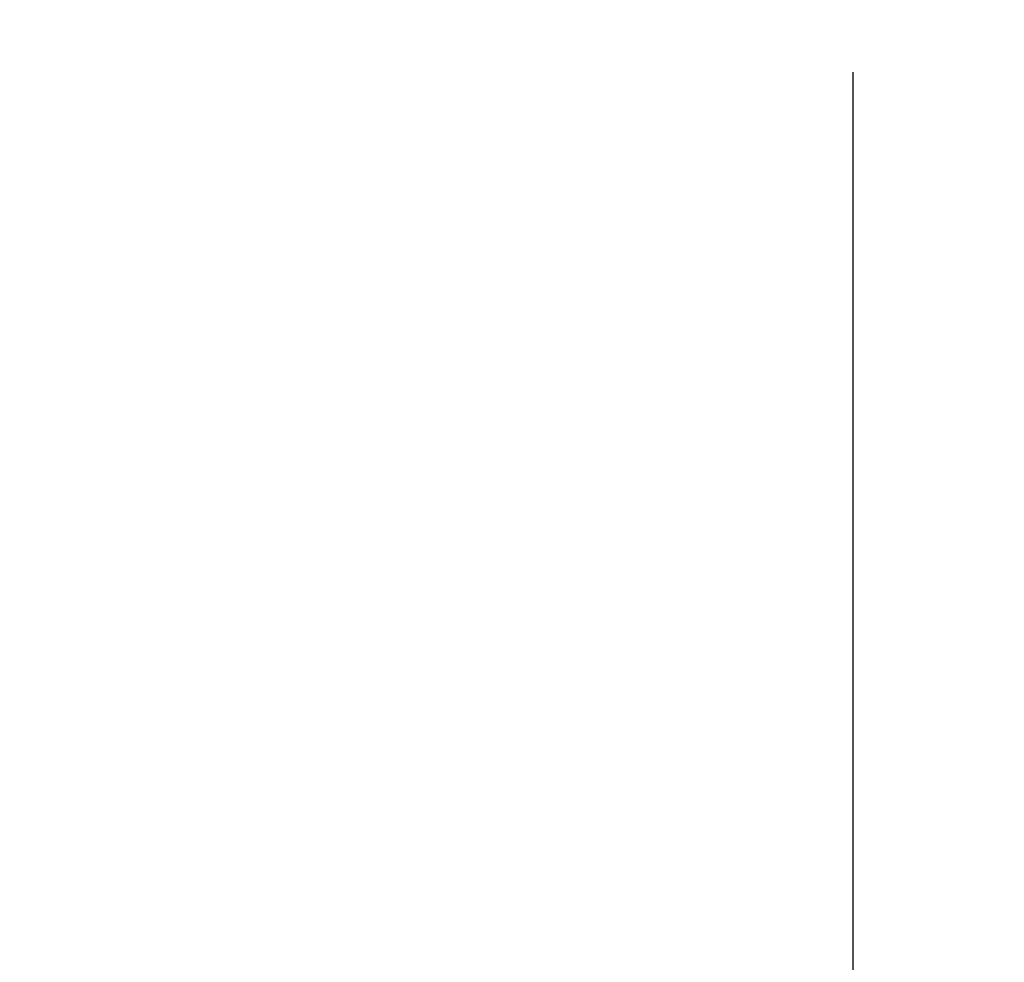
# Model space of a CAD drawing. Units: inches. Extents: x 2083 to 3317, y 1141 to 2115.
# Tile 126 of 256: x 3119.674 to 3128.284, y 1254.858 to 1263.096. Entities that reach past the tile are written whole.
import ezdxf

# ---------------------------------------------------------------- set-up
doc = ezdxf.new("R2010")
doc.units = ezdxf.units.IN
doc.layers.add('A-ANNO-DIMS', color=2, linetype='Continuous', lineweight=18)
doc.styles.get("Standard").update_dxf_attribs({"font": 'arial.ttf'})
doc.dimstyles.new('ISO-25', dxfattribs={"dimtxt": 12, "dimasz": 12, "dimexe": 1.25, "dimexo": 0.625, "dimtad": 1, "dimlunit": 3, "dimtxsty": 'Standard', "dimcen": 2.5, "dimadec": 0, "dimazin": 0, "dimtfac": 1, "dimtmove": 0, "dimatfit": 3, "dimfxl": 1, "dimarcsym": 0})

# ---------------------------------------------------------------- blocks, each defined once
blk = doc.blocks.new('*D10')
at = {"layer": 'A-ANNO-DIMS', "color": 0, "lineweight": -2, "transparency": 16777216}
for p, q in [((2862.9598, 1262.6364), (2862.9598, 1201.3844)), ((3126.9598, 1262.6364), (3126.9598, 1201.3844)), ((2874.9598, 1202.6344), (3114.9598, 1202.6344))]:
    blk.add_line(p, q, dxfattribs=at)
at = {"layer": 'A-ANNO-DIMS', "color": 0, "transparency": 16777216}
for points in [[(2874.9598, 1204.6344), (2874.9598, 1200.6344), (2862.9598, 1202.6344)], [(3114.9598, 1204.6344), (3114.9598, 1200.6344), (3126.9598, 1202.6344)]]:
    blk.add_solid(points, dxfattribs=at)
at = {"layer": 'Defpoints', "color": 0, "transparency": 16777216}
for p in [(2862.9598, 1263.2614), (3126.9598, 1263.2614), (3126.9598, 1202.6344)]:
    blk.add_point(p, dxfattribs=at)
at = {"layer": 'A-ANNO-DIMS', "color": 0, "transparency": 16777216, "insert": (2994.9598, 1209.284), "char_height": 12, "attachment_point": 5}
blk.add_mtext("22'", dxfattribs=at)
blk = doc.blocks.new('*D26')
at = {"layer": 'A-ANNO-DIMS', "color": 0, "lineweight": -2, "transparency": 16777216}
for p, q in [((3088.9858, 1274.9151), (3088.9858, 1270.952)), ((3111.24, 1274.9151), (3111.24, 1270.952)), ((3076.9858, 1272.202), (2840.2624, 1272.202)), ((3111.24, 1272.202), (3088.9858, 1272.202)), ((3123.24, 1272.202), (3135.24, 1272.202))]:
    blk.add_line(p, q, dxfattribs=at)
at = {"layer": 'A-ANNO-DIMS', "color": 0, "transparency": 16777216}
for points in [[(3076.9858, 1274.202), (3076.9858, 1270.202), (3088.9858, 1272.202)], [(3123.24, 1274.202), (3123.24, 1270.202), (3111.24, 1272.202)]]:
    blk.add_solid(points, dxfattribs=at)
at = {"layer": 'Defpoints', "color": 0, "transparency": 16777216}
for p in [(3088.9858, 1275.5401), (3111.24, 1275.5401), (3088.9858, 1272.202)]:
    blk.add_point(p, dxfattribs=at)
at = {"layer": 'A-ANNO-DIMS', "color": 0, "transparency": 16777216, "insert": (2952.6241, 1279.0316), "char_height": 12, "attachment_point": 5}
blk.add_mtext('NIGHTSTAND 1\'-10 1/2" TYP.', dxfattribs=at)
blk = doc.blocks.new('*D27')
at = {"layer": 'A-ANNO-DIMS', "color": 0, "lineweight": -2, "transparency": 16777216}
for p, q in [((3114.5782, 1309.7943), (3114.5782, 1321.7943)), ((3111.865, 1297.7943), (3115.8282, 1297.7943)), ((3114.5782, 1297.7943), (3114.5782, 1275.5401)), ((3111.865, 1275.5401), (3115.8282, 1275.5401)), ((3114.5782, 1263.5401), (3114.5782, 1140.9886))]:
    blk.add_line(p, q, dxfattribs=at)
at = {"layer": 'A-ANNO-DIMS', "color": 0, "transparency": 16777216}
for points in [[(3112.5782, 1309.7943), (3116.5782, 1309.7943), (3114.5782, 1297.7943)], [(3112.5782, 1263.5401), (3116.5782, 1263.5401), (3114.5782, 1275.5401)]]:
    blk.add_solid(points, dxfattribs=at)
at = {"layer": 'Defpoints', "color": 0, "transparency": 16777216}
for p in [(3111.24, 1297.7943), (3111.24, 1275.5401), (3114.5782, 1275.5401)]:
    blk.add_point(p, dxfattribs=at)
at = {"layer": 'A-ANNO-DIMS', "color": 0, "transparency": 16777216, "insert": (3107.7485, 1196.2643), "char_height": 12, "attachment_point": 5, "rotation": 90}
blk.add_mtext('1\'-10 1/2" TYP.', dxfattribs=at)
blk = doc.blocks.new('*D34')
at = {"layer": 'A-ANNO-DIMS', "color": 0, "lineweight": -2, "transparency": 16777216}
for p, q in [((2226.9598, 1262.6364), (2226.9598, 1209.6614)), ((3126.9598, 1262.6364), (3126.9598, 1209.6614)), ((2238.9598, 1210.9114), (3114.9598, 1210.9114))]:
    blk.add_line(p, q, dxfattribs=at)
at = {"layer": 'A-ANNO-DIMS', "color": 0, "transparency": 16777216}
for points in [[(2238.9598, 1212.9114), (2238.9598, 1208.9114), (2226.9598, 1210.9114)], [(3114.9598, 1212.9114), (3114.9598, 1208.9114), (3126.9598, 1210.9114)]]:
    blk.add_solid(points, dxfattribs=at)
at = {"layer": 'Defpoints', "color": 0, "transparency": 16777216}
for p in [(2226.9598, 1263.2614), (3126.9598, 1263.2614), (3126.9598, 1210.9114)]:
    blk.add_point(p, dxfattribs=at)
at = {"layer": 'A-ANNO-DIMS', "color": 0, "transparency": 16777216, "insert": (2676.9598, 1217.6632), "char_height": 12, "attachment_point": 5}
blk.add_mtext('75\'-0"', dxfattribs=at)

msp = doc.modelspace()

# ---------------------------------------------------------------- dimensions: what is measured, and where the dimension line sits
at = {"layer": 'A-ANNO-DIMS'}
for base, p1, p2, angle, text, picture, middle in [((3114.5782, 1275.5401), (3111.24, 1297.7943), (3111.24, 1275.5401), 270, '<> TYP.', '*D27', (3107.7485, 1196.2643)), ((3088.9858, 1272.202), (3111.24, 1275.5401), (3088.9858, 1275.5401), 180, 'NIGHTSTAND <> TYP.', '*D26', (2952.6241, 1279.0316))]:
    dim = msp.add_linear_dim(base=base, p1=p1, p2=p2, angle=angle, text=text, dimstyle='ISO-25', override={"dimdec": 1, "dimlfac": 1, "dimrnd": 0, "dimzin": 1, "dimdsep": 46, "dimlunit": 4, "dimfrac": 2}, dxfattribs=at)
    dim.commit()
    dim.dimension.update_dxf_attribs({"geometry": picture, "text_midpoint": middle})
for base, p1, override, picture, middle in [((3126.9598, 1210.9114), (2226.9598, 1263.2614), {"dimdec": 1, "dimlfac": 1, "dimrnd": 0, "dimzin": 1, "dimdsep": 46, "dimlunit": 4, "dimfrac": 2}, '*D34', (2676.9598, 1217.6632)), ((3126.9598, 1202.6344), (2862.9598, 1263.2614), {"dimclrd": 0, "dimclre": 0, "dimclrt": 0}, '*D10', (2994.9598, 1209.284))]:
    dim = msp.add_linear_dim(base=base, p1=p1, p2=(3126.9598, 1263.2614), dimstyle='ISO-25', override=override, dxfattribs=at)
    dim.commit()
    dim.dimension.update_dxf_attribs({"geometry": picture, "text_midpoint": middle})

doc.saveas('drawing.dxf')
